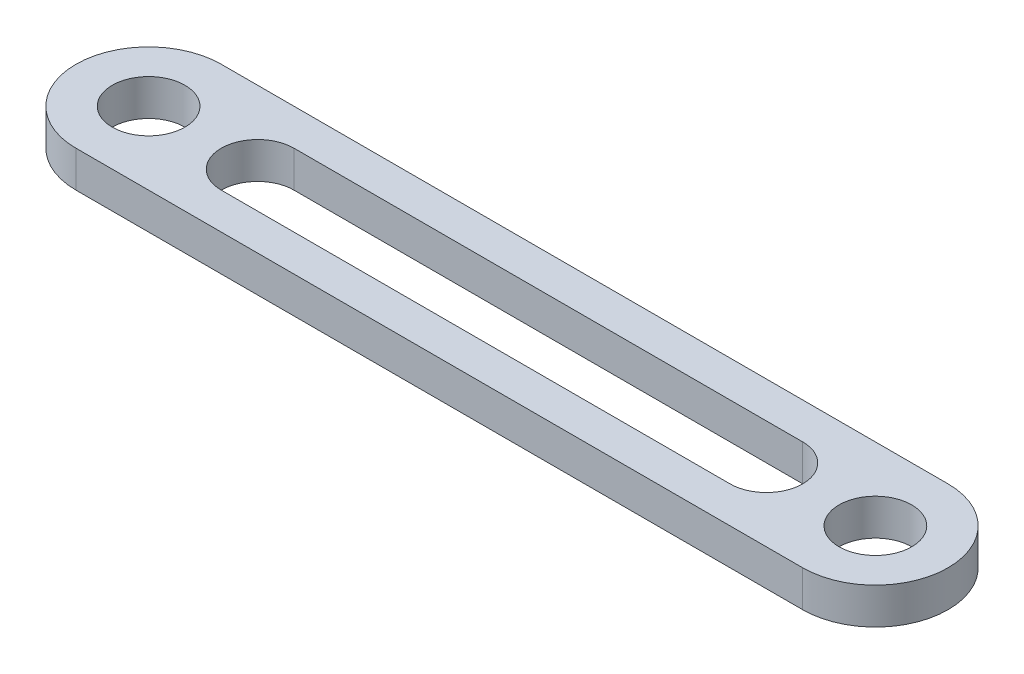
SolidWorks part; units mm, degrees
material "Plain Carbon Steel"
ref_plane "Front Plane" through (0, 0, 0) normal (0, 0, 1) x (1, 0, 0)
ref_plane "Top Plane" through (0, 0, 0) normal (0, 1, 0) x (1, 0, 0)
ref_plane "Right Plane" through (0, 0, 0) normal (1, 0, 0) x (0, 0, -1)
sketch "Link Profile Sketch" plane through (0, 0, 0) normal (0, 1, 0) x (1, 0, 0)
  line L0 (-50, 0) -> (50, 0) construction
  line L1 (-50, 10) -> (50, 10)
  line L2 (-50, -10) -> (50, -10)
  line L3 (-35, 0) -> (35, 0) construction
  line L4 (-35, 5) -> (35, 5)
  line L5 (-35, -5) -> (35, -5)
  arc A0 (-50, 10) -> (-50, -10) centre (-50, 0) ccw
  arc A1 (50, -10) -> (50, 10) centre (50, 0) ccw
  circle A2 centre (-50, 0) radius 5
  circle A3 centre (50, 0) radius 5
  arc A4 (-35, 5) -> (-35, -5) centre (-35, 0) ccw
  arc A5 (35, -5) -> (35, 5) centre (35, 0) ccw
  point P2 (0, 0)
  point P14 (0, 0)
  dimension "D1" = 10
  dimension "D3" = 10
  dimension "D4" = 10
  dimension "D5" = 5
  dimension "D2" = 100
  dimension "D6" = 15
extrude "Link Plate 5mm" add sketch "Link Profile Sketch" along normal blind 5
